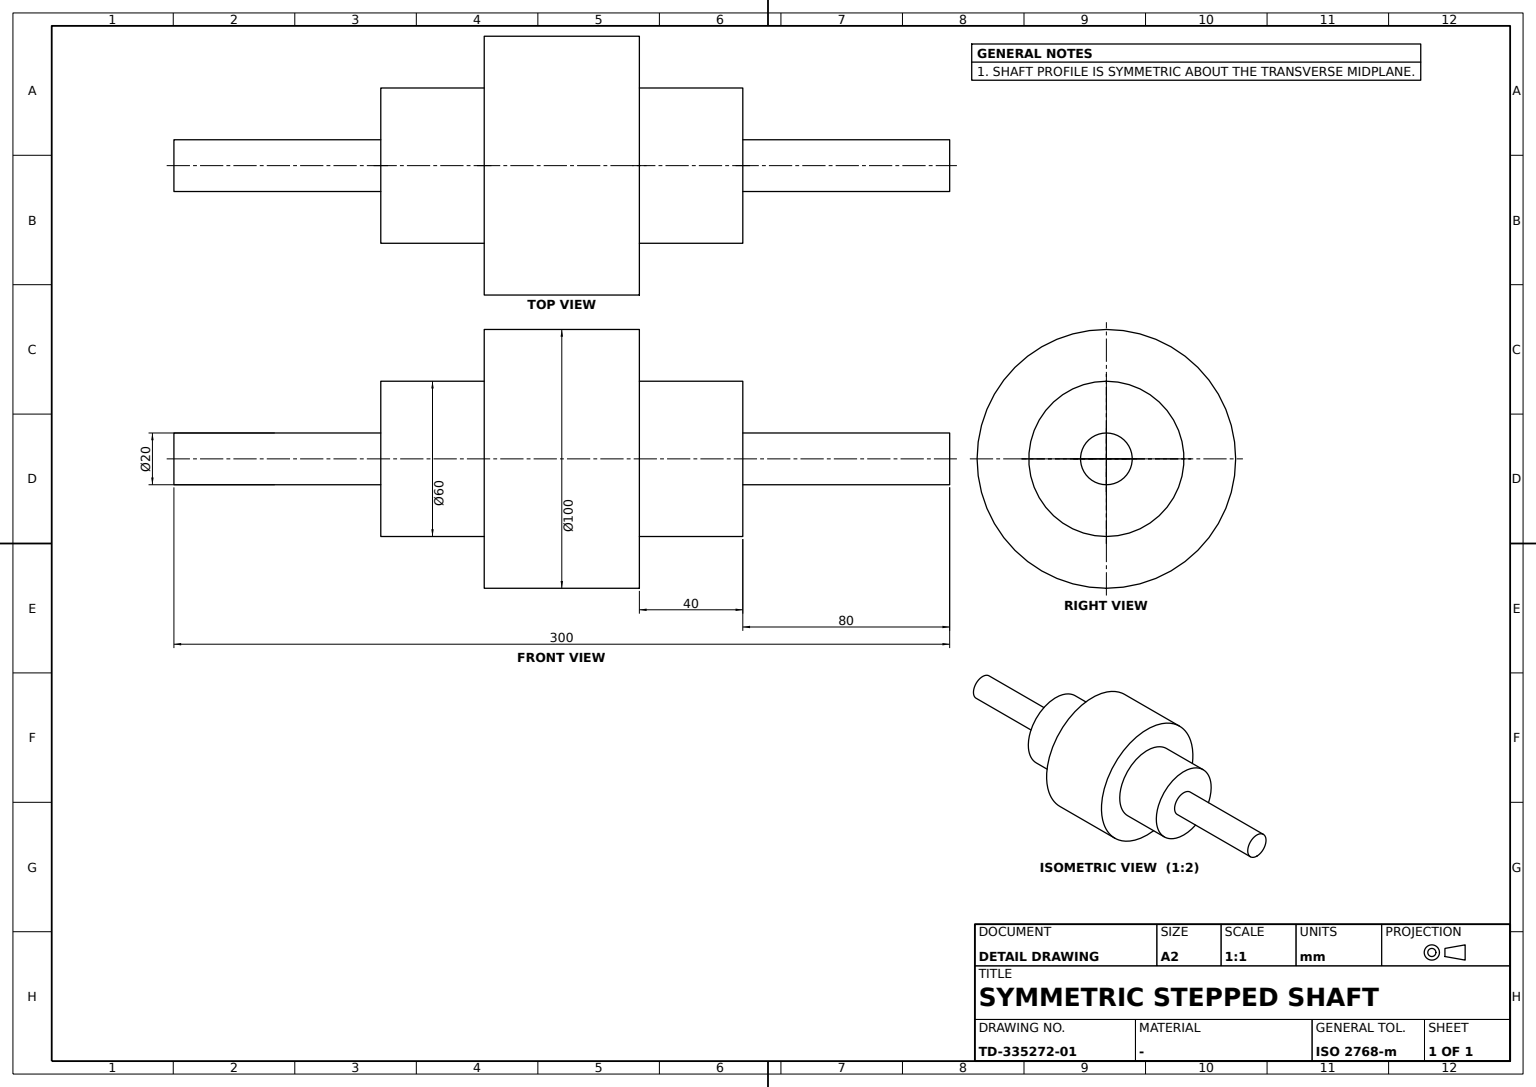
CATIA V5 part; units mm, degrees
sketch "Sketch1" plane through (0, 0, 0) normal (-1, 0, 0) x (0, -1, 0)
  line L0 (0, 0) -> (0, 10)
  line L1 (0, 10) -> (80, 10)
  line L2 (80, 10) -> (80, 30)
  line L3 (80, 30) -> (120, 30)
  line L4 (120, 30) -> (120, 50)
  line L5 (120, 50) -> (180, 50)
  line L6 (180, 50) -> (180, 30)
  point P0 (180, 30)
  line L7 (180, 30) -> (220, 30)
  line L8 (220, 30) -> (220, 10)
  line L9 (220, 10) -> (300, 10)
  line L10 (300, 10) -> (300, 0)
  point P1 (300, 0)
  line L11 (300, 0) -> (0, 0)
  dimension "length L11" = 300
  dimension "length L2" = 20
  dimension "length L0" = 10
  dimension "length L4" = 20
  dimension "length L3" = 40
  dimension "length L1" = 80
  dimension "length L10" = 10
  dimension "length L7" = 40
  dimension "length L9" = 80
  constraint vertical L0 y-axis
  constraint vertical L2 y-axis
  constraint vertical L4 y-axis
  constraint vertical L6 y-axis
  constraint vertical L8 y-axis
  constraint vertical L10 y-axis
  constraint horizontal L1 x-axis
  constraint horizontal L3 x-axis
  constraint horizontal L5 x-axis
  constraint horizontal L7 x-axis
  constraint horizontal L9 x-axis
  constraint horizontal L11 x-axis
  constraint coincidence P0 L3
  constraint coincidence P1 x-axis
revolve "Shaft1" add sketch "Sketch1" angle 360 about L11
properties part number "p5"
